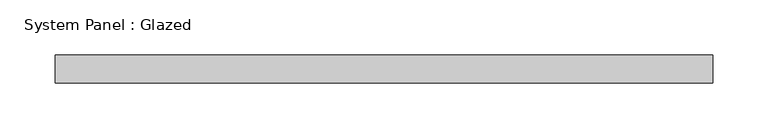
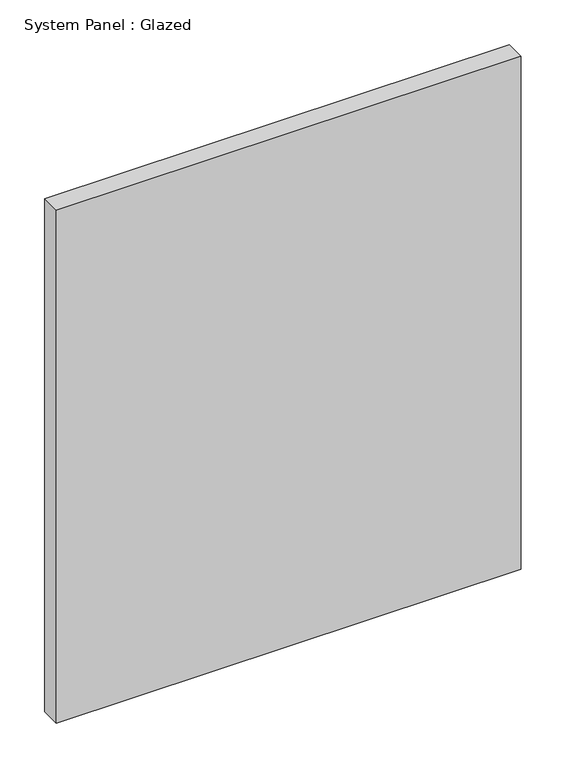
"""IFC4 building model written with IfcOpenShell, lengths in millimetres: plate geometry, System Panel : Glazed."""

from ifc_helpers import new_model, si_unit, origin, origin_with_axes, place, context, project, spatial, polyline, outline, extrude, source, transform, mapped, element, save


def system_panel_glazed_89c3752f(model_context):
    return source(origin(), model_context, "Body", "SweptSolid", [
        extrude(outline(polyline([(298.45, 19.05), (-298.45, 19.05), (-298.45, 44.45), (298.45, 44.45), (298.45, 19.05)])), origin_with_axes(), (0.0, 0.0, 1.0), 696.0441631),
    ])


if __name__ == "__main__":
    model = new_model("IFC4")
    model_context = context("Model", 3, world=origin())
    ifc_project = project(units=[si_unit("LENGTHUNIT", "METRE", prefix="MILLI")], contexts=[model_context])
    site = spatial("IfcSite", under=ifc_project)
    building = spatial("IfcBuilding", under=site)
    placement = place(None, origin())
    system_panel_glazed_shape = system_panel_glazed_89c3752f(model_context)
    element("IfcPlate", 1, ObjectType="System Panel : Glazed", at=placement, inside=building, context=model_context, shape_type="MappedRepresentation", body=[
        mapped(system_panel_glazed_shape, transform((0.0, 0.0, 0.0), x_axis=(1.0, 0.0, 0.0), y_axis=(0.0, 1.0, 0.0), z_axis=(0.0, 0.0, 1.0))),
    ])
    save(model, "model.ifc")

# Revit data of these elements
# Type "System Panel : Glazed"
#   Construction Type Id = "GSP4R"
#   Analytic Construction = "1/8 in Pilkington single glazing"
#   Visual Light Transmittance = 0.9
#   Solar Heat Gain Coefficient = 0.86
#   Heat Transfer Coefficient (U) = 1.18115 BTU/(h·ft²·°F)
#   Define Thermal Properties by = 1
# Element 1 (IfcPlate, "System Panel : Glazed")
#   Materials on its faces: "Glass"
# Materials
#   "Glass": class "Glass", colour RGB 0 128 192, transparency 0.75, Description = "Soda Lime Glass", Cost = 0
